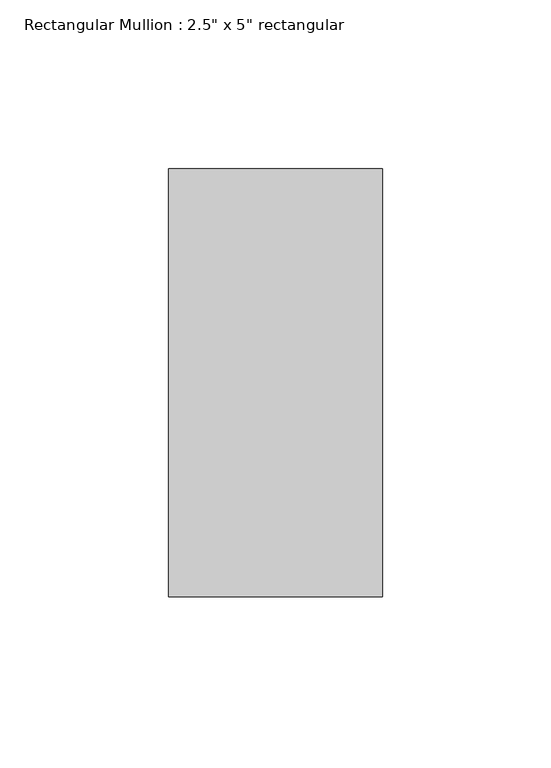
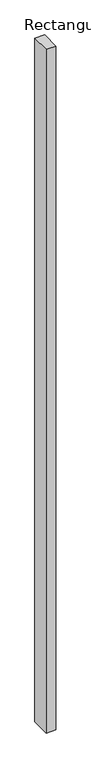
"""IFC4 building model written with IfcOpenShell, lengths in millimetres: member geometry."""

from ifc_helpers import new_model, si_unit, frame, origin, place, context, project, spatial, polyline, outline, extrude, source, transform, mapped, element, save


def member_e4af79e9(model_context):
    return source(origin(), model_context, "Body", "SweptSolid", [
        extrude(outline(polyline([(0.0, 63.5), (0.0, -63.5), (-63.5, -63.5), (-63.5, 63.5), (0.0, 63.5)])), frame((0.0, 0.0, -4711.7), z_axis=(0.0, 0.0, 1.0), x_axis=(1.0, 0.0, 0.0)), (0.0, 0.0, 1.0), 4711.7),
    ])


if __name__ == "__main__":
    model = new_model("IFC4")
    model_context = context("Model", 3, world=origin())
    ifc_project = project(units=[si_unit("LENGTHUNIT", "METRE", prefix="MILLI")], contexts=[model_context])
    site = spatial("IfcSite", under=ifc_project)
    building = spatial("IfcBuilding", under=site)
    placement = place(None, origin())
    member_shape = member_e4af79e9(model_context)
    element("IfcMember", 1, ObjectType="Rectangular Mullion : 2.5\" x 5\" rectangular", at=placement, inside=building, context=model_context, shape_type="MappedRepresentation", body=[
        mapped(member_shape, transform((0.0, 0.0, 0.0), x_axis=(1.0, 0.0, 0.0), y_axis=(0.0, 1.0, 0.0), z_axis=(0.0, 0.0, 1.0))),
    ])
    save(model, "model.ifc")

# Revit data of these elements
# Type "Rectangular Mullion : 2.5\" x 5\" rectangular"
#   built-in parameter 1007304 = 0.416667 (stored number, unit not read)
#   built-in parameter 1007301 = 0.104167 (stored number, unit not read)
#   built-in parameter 1007300 = 0.104167 (stored number, unit not read)
# Element 1 (IfcMember, "Rectangular Mullion : 2.5\" x 5\" rectangular")
#   Materials on its faces: "Aluminum"
# Materials
#   "Aluminum": class "Metal", colour RGB 247 247 247, transparency 0, Description = "Aluminum 6061", Cost = 0
